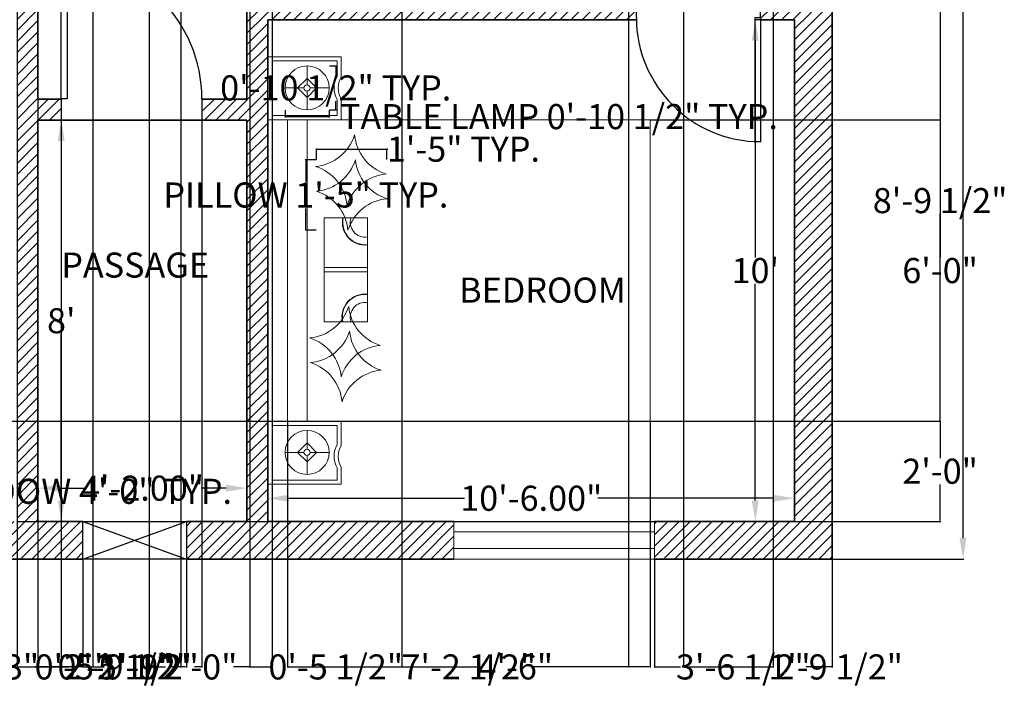
# Model space of a CAD drawing. Units: inches. Extents: x -302 to 383, y -29 to 550.
# Tile 2 of 4: x 147 to 383, y -14 to 149. Entities that reach past the tile are written whole.
import ezdxf

# ---------------------------------------------------------------- set-up
doc = ezdxf.new("R2010")
doc.units = ezdxf.units.IN
doc.header["$MEASUREMENT"] = 0
for name, color, linetype, lineweight in [('A-ANNO-DIMS', 3, 'Continuous', 18), ('A-AREA-IDEN', 2, 'Continuous', 25), ('A-DOOR', 4, 'Continuous', 25), ('A-FURN', 1, 'Continuous', 18), ('A-GLAZ', 2, 'Continuous', 18), ('A-WALL', 7, 'Continuous', 35), ('A-WALL-PATT', 252, 'Continuous', 13)]:
    doc.layers.add(name, color=color, linetype=linetype, lineweight=lineweight)
doc.styles.get("Standard").update_dxf_attribs({"font": 'arial.ttf'})
doc.dimstyles.get("Standard").update_dxf_attribs({"dimtxt": 6, "dimasz": 0.18, "dimexe": 0.18, "dimexo": 0.0625, "dimgap": 0.09, "dimtad": 0, "dimtih": 1, "dimtoh": 1, "dimzin": 0, "dimdsep": 46, "dimlunit": 3, "dimtxsty": 'Standard', "dimcen": 0.09, "dimadec": 0, "dimazin": 0, "dimtfac": 1, "dimtofl": 0, "dimtmove": 0, "dimatfit": 3, "dimfxl": 1, "dimtolj": 1, "dimtzin": 0, "dimarcsym": 0})

# ---------------------------------------------------------------- blocks, each defined once
blk = doc.blocks.new('*U2')
for p, q in [((0, 0), (0, -6)), ((40, 0), (40, -6))]:
    blk.add_line(p, q)
blk.add_lwpolyline([(0, 0), (0, 40), (1.75, 40), (1.75, 0)], close=True)
blk.add_arc((0, 0), 40, 0, 90)
blk = doc.blocks.new('Lamp - Table')
for p, q in [((0, 7), (0, 1)), ((-1, 0), (-7, 0)), ((0, 3), (-3, 0)), ((-3, 0), (0, -3)), ((3, 0), (0, 3)), ((0, -3), (3, 0)), ((1, 0), (7, 0)), ((0, -1), (0, -7))]:
    blk.add_line(p, q)
for radius in [7, 1]:
    blk.add_circle((0, 0), radius)
blk = doc.blocks.new('*D15')
at = {"layer": 'A-ANNO-DIMS', "color": 0, "lineweight": -2, "transparency": 16777216}
for p, q in [((206.7, 29.34), (206.7, 34.99)), ((211.7, 34.81), (253.76, 34.81)), ((327.7, 34.81), (285.64, 34.81)), ((332.7, 29.34), (332.7, 34.99))]:
    blk.add_line(p, q, dxfattribs=at)
at = {"layer": 'A-ANNO-DIMS', "color": 0, "transparency": 16777216}
for points in [[(211.7, 35.64), (211.7, 33.98), (206.7, 34.81)], [(327.7, 35.64), (327.7, 33.98), (332.7, 34.81)]]:
    blk.add_solid(points, dxfattribs=at)
at = {"layer": 'Defpoints', "color": 0, "transparency": 16777216}
for p in [(332.7, 34.81), (206.7, 29.27), (332.7, 29.27)]:
    blk.add_point(p, dxfattribs=at)
at = {"layer": 'A-ANNO-DIMS', "color": 0, "transparency": 16777216, "insert": (269.7, 34.81), "char_height": 6, "attachment_point": 5}
blk.add_mtext('\\A1;10\'-6.00"', dxfattribs=at)
blk = doc.blocks.new('*D16')
at = {"layer": 'A-ANNO-DIMS', "color": 0, "lineweight": -2, "transparency": 16777216}
for p, q in [((332.63, 149.27), (323.11, 149.27)), ((323.29, 144.27), (323.29, 92.43)), ((323.29, 34.27), (323.29, 86.12)), ((332.63, 29.27), (323.11, 29.27))]:
    blk.add_line(p, q, dxfattribs=at)
at = {"layer": 'A-ANNO-DIMS', "color": 0, "transparency": 16777216}
for points in [[(322.45, 144.27), (324.12, 144.27), (323.29, 149.27)], [(322.45, 34.27), (324.12, 34.27), (323.29, 29.27)]]:
    blk.add_solid(points, dxfattribs=at)
at = {"layer": 'Defpoints', "color": 0, "transparency": 16777216}
for p in [(332.7, 149.27), (323.29, 29.27), (332.7, 29.27)]:
    blk.add_point(p, dxfattribs=at)
at = {"layer": 'A-ANNO-DIMS', "color": 0, "transparency": 16777216, "insert": (323.29, 89.27), "char_height": 6, "attachment_point": 5}
blk.add_mtext("\\A1;10'", dxfattribs=at)
blk = doc.blocks.new('*D17')
at = {"layer": 'A-ANNO-DIMS', "color": 0, "lineweight": -2, "transparency": 16777216}
for p, q in [((151.7, 29.34), (151.7, 37.4)), ((156.7, 37.22), (162.69, 37.22)), ((196.7, 37.22), (190.71, 37.22)), ((201.7, 29.34), (201.7, 37.4))]:
    blk.add_line(p, q, dxfattribs=at)
at = {"layer": 'A-ANNO-DIMS', "color": 0, "transparency": 16777216}
for points in [[(156.7, 38.06), (156.7, 36.39), (151.7, 37.22)], [(196.7, 38.06), (196.7, 36.39), (201.7, 37.22)]]:
    blk.add_solid(points, dxfattribs=at)
at = {"layer": 'Defpoints', "color": 0, "transparency": 16777216}
for p in [(201.7, 37.22), (151.7, 29.27), (201.7, 29.27)]:
    blk.add_point(p, dxfattribs=at)
at = {"layer": 'A-ANNO-DIMS', "color": 0, "transparency": 16777216, "insert": (176.7, 37.22), "char_height": 6, "attachment_point": 5}
blk.add_mtext('\\A1;4\'-2.00"', dxfattribs=at)
blk = doc.blocks.new('*D18')
at = {"layer": 'A-ANNO-DIMS', "color": 0, "lineweight": -2, "transparency": 16777216}
for p, q in [((151.76, 125.27), (157.46, 125.27)), ((157.28, 120.27), (157.28, 80.43)), ((157.28, 34.27), (157.28, 74.12)), ((151.76, 29.27), (157.46, 29.27))]:
    blk.add_line(p, q, dxfattribs=at)
at = {"layer": 'A-ANNO-DIMS', "color": 0, "transparency": 16777216}
for points in [[(156.45, 120.27), (158.11, 120.27), (157.28, 125.27)], [(156.45, 34.27), (158.11, 34.27), (157.28, 29.27)]]:
    blk.add_solid(points, dxfattribs=at)
at = {"layer": 'Defpoints', "color": 0, "transparency": 16777216}
for p in [(151.7, 125.27), (151.7, 29.27), (157.28, 29.27)]:
    blk.add_point(p, dxfattribs=at)
at = {"layer": 'A-ANNO-DIMS', "color": 0, "transparency": 16777216, "insert": (157.28, 77.27), "char_height": 6, "attachment_point": 5}
blk.add_mtext("\\A1;8'", dxfattribs=at)
blk = doc.blocks.new('*D22')
at = {"layer": 'A-ANNO-DIMS', "color": 0, "lineweight": -2, "transparency": 16777216}
for p, q in [((341.76, 464.27), (373.16, 464.27)), ((372.98, 459.27), (372.98, 245.43)), ((372.98, 25.27), (372.98, 239.12)), ((341.76, 20.27), (373.16, 20.27))]:
    blk.add_line(p, q, dxfattribs=at)
at = {"layer": 'A-ANNO-DIMS', "color": 0, "transparency": 16777216}
for points in [[(372.15, 459.27), (373.82, 459.27), (372.98, 464.27)], [(372.15, 25.27), (373.82, 25.27), (372.98, 20.27)]]:
    blk.add_solid(points, dxfattribs=at)
at = {"layer": 'Defpoints', "color": 0, "transparency": 16777216}
for p in [(341.7, 464.27), (341.7, 20.27), (372.98, 20.27)]:
    blk.add_point(p, dxfattribs=at)
at = {"layer": 'A-ANNO-DIMS', "color": 0, "transparency": 16777216, "insert": (372.98, 242.27), "char_height": 6, "attachment_point": 5}
blk.add_mtext("\\A1;37'", dxfattribs=at)
blk = doc.blocks.new('WIN-48IN')
blk.add_lwpolyline([(0, 9), (48, 9), (48, 0), (0, 0)], close=True)
for points in [[(0, 6.5), (48, 6.5)], [(0, 2.5), (48, 2.5)]]:
    blk.add_lwpolyline(points)
blk = doc.blocks.new('BED-THROW-PILLOW')
for centre, start, end in [((2.25, 23.4), 275.3318, 342.5062), ((23.4, 21.14), 185.3318, 252.5062), ((0, 2.25), 5.3318, 72.5062), ((21.14, 0), 95.3318, 162.5062)]:
    blk.add_arc(centre, 10.85, start, end)
blk = doc.blocks.new('*D29')
at = {"layer": 'A-ANNO-DIMS', "color": 0, "lineweight": -2, "transparency": 16777216}
for p, q in [((75.47, 29.34), (75.47, 36.65)), ((75.65, 36.47), (123.29, 36.47)), ((123.47, 29.34), (123.47, 36.65)), ((123.47, 36.47), (123.65, 36.47))]:
    blk.add_line(p, q, dxfattribs=at)
at = {"layer": 'A-ANNO-DIMS', "color": 0, "transparency": 16777216}
for points in [[(75.65, 36.5), (75.65, 36.44), (75.47, 36.47)], [(123.29, 36.5), (123.29, 36.44), (123.47, 36.47)]]:
    blk.add_solid(points, dxfattribs=at)
at = {"layer": 'Defpoints', "color": 0, "transparency": 16777216}
for p in [(123.47, 36.47), (75.47, 29.27), (123.47, 29.27)]:
    blk.add_point(p, dxfattribs=at)
at = {"layer": 'A-ANNO-DIMS', "color": 0, "transparency": 16777216, "insert": (161.7, 36.47), "char_height": 6, "attachment_point": 5}
blk.add_mtext('\\A1;WINDOW 4\'-0" TYP.', dxfattribs=at)
blk = doc.blocks.new('*D33')
at = {"layer": 'A-ANNO-DIMS', "color": 0, "lineweight": -2, "transparency": 16777216}
for p, q in [((210.8, 127.61), (210.8, 125.91)), ((221.35, 127.61), (221.35, 125.91)), ((210.98, 126.09), (221.17, 126.09)), ((221.35, 126.09), (221.53, 126.09))]:
    blk.add_line(p, q, dxfattribs=at)
at = {"layer": 'A-ANNO-DIMS', "color": 0, "transparency": 16777216}
for points in [[(210.98, 126.12), (210.98, 126.06), (210.8, 126.09)], [(221.17, 126.12), (221.17, 126.06), (221.35, 126.09)]]:
    blk.add_solid(points, dxfattribs=at)
at = {"layer": 'Defpoints', "color": 0, "transparency": 16777216}
for p in [(210.8, 127.68), (221.35, 127.68), (221.35, 126.09)]:
    blk.add_point(p, dxfattribs=at)
at = {"layer": 'A-ANNO-DIMS', "color": 0, "transparency": 16777216, "insert": (276.32, 126.09), "char_height": 6, "attachment_point": 5}
blk.add_mtext('\\A1;TABLE LAMP 0\'-10 1/2" TYP.', dxfattribs=at)
blk = doc.blocks.new('*D34')
at = {"layer": 'A-ANNO-DIMS', "color": 0, "lineweight": -2, "transparency": 16777216}
for p, q in [((221.41, 138.22), (223.11, 138.22)), ((222.93, 138.04), (222.93, 136.14)), ((222.93, 127.86), (222.93, 129.76)), ((221.41, 127.68), (223.11, 127.68))]:
    blk.add_line(p, q, dxfattribs=at)
at = {"layer": 'A-ANNO-DIMS', "color": 0, "transparency": 16777216}
for points in [[(222.9, 138.04), (222.96, 138.04), (222.93, 138.22)], [(222.9, 127.86), (222.96, 127.86), (222.93, 127.68)]]:
    blk.add_solid(points, dxfattribs=at)
at = {"layer": 'Defpoints', "color": 0, "transparency": 16777216}
for p in [(221.35, 138.22), (222.93, 138.22), (221.35, 127.68)]:
    blk.add_point(p, dxfattribs=at)
at = {"layer": 'A-ANNO-DIMS', "color": 0, "transparency": 16777216, "insert": (222.93, 132.95), "char_height": 6, "attachment_point": 5}
blk.add_mtext('\\A1;0\'-10 1/2" TYP.', dxfattribs=at)
blk = doc.blocks.new('*D35')
at = {"layer": 'A-ANNO-DIMS', "color": 0, "lineweight": -2, "transparency": 16777216}
for p, q in [((218.26, 115.78), (215.61, 115.78)), ((215.79, 115.6), (215.79, 110.54)), ((215.79, 99.08), (215.79, 104.15)), ((218.26, 98.9), (215.61, 98.9))]:
    blk.add_line(p, q, dxfattribs=at)
at = {"layer": 'A-ANNO-DIMS', "color": 0, "transparency": 16777216}
for points in [[(215.76, 115.6), (215.82, 115.6), (215.79, 115.78)], [(215.76, 99.08), (215.82, 99.08), (215.79, 98.9)]]:
    blk.add_solid(points, dxfattribs=at)
at = {"layer": 'Defpoints', "color": 0, "transparency": 16777216}
for p in [(215.79, 115.78), (218.32, 115.78), (218.32, 98.9)]:
    blk.add_point(p, dxfattribs=at)
at = {"layer": 'A-ANNO-DIMS', "color": 0, "transparency": 16777216, "insert": (215.79, 107.34), "char_height": 6, "attachment_point": 5}
blk.add_mtext('\\A1;PILLOW 1\'-5" TYP.', dxfattribs=at)
blk = doc.blocks.new('*D36')
at = {"layer": 'A-ANNO-DIMS', "color": 0, "lineweight": -2, "transparency": 16777216}
for p, q in [((218.32, 115.84), (218.32, 118.49)), ((218.5, 118.31), (235.01, 118.31)), ((235.19, 115.84), (235.19, 118.49)), ((235.19, 118.31), (235.37, 118.31))]:
    blk.add_line(p, q, dxfattribs=at)
at = {"layer": 'A-ANNO-DIMS', "color": 0, "transparency": 16777216}
for points in [[(218.5, 118.34), (218.5, 118.28), (218.32, 118.31)], [(235.01, 118.34), (235.01, 118.28), (235.19, 118.31)]]:
    blk.add_solid(points, dxfattribs=at)
at = {"layer": 'Defpoints', "color": 0, "transparency": 16777216}
for p in [(235.19, 118.31), (218.32, 115.78), (235.19, 115.78)]:
    blk.add_point(p, dxfattribs=at)
at = {"layer": 'A-ANNO-DIMS', "color": 0, "transparency": 16777216, "insert": (253.47, 118.31), "char_height": 6, "attachment_point": 5}
blk.add_mtext('\\A1;1\'-5" TYP.', dxfattribs=at)
blk = doc.blocks.new('*D38')
at = {"layer": 'A-ANNO-DIMS', "color": 0, "lineweight": -2, "transparency": 16777216}
for p, q in [((123.47, 20.21), (123.47, -5.71)), ((162.44, 20.21), (162.44, -5.71)), ((123.65, -5.53), (134.89, -5.53)), ((162.26, -5.53), (151.02, -5.53))]:
    blk.add_line(p, q, dxfattribs=at)
at = {"layer": 'A-ANNO-DIMS', "color": 0, "transparency": 16777216}
for points in [[(123.65, -5.5), (123.65, -5.56), (123.47, -5.53)], [(162.26, -5.5), (162.26, -5.56), (162.44, -5.53)]]:
    blk.add_solid(points, dxfattribs=at)
at = {"layer": 'Defpoints', "color": 0, "transparency": 16777216}
for p in [(123.47, 20.27), (162.44, 20.27), (162.44, -5.53)]:
    blk.add_point(p, dxfattribs=at)
at = {"layer": 'A-ANNO-DIMS', "color": 0, "transparency": 16777216, "insert": (142.95, -5.53), "char_height": 6, "attachment_point": 5}
blk.add_mtext('\\A1;3\'-3"', dxfattribs=at)
blk = doc.blocks.new('*D39')
at = {"layer": 'A-ANNO-DIMS', "color": 0, "lineweight": -2, "transparency": 16777216}
for p, q in [((162.44, 20.21), (162.44, -5.71)), ((187.2, 20.21), (187.2, -5.71)), ((162.62, -5.53), (166.7, -5.53)), ((187.02, -5.53), (182.94, -5.53))]:
    blk.add_line(p, q, dxfattribs=at)
at = {"layer": 'A-ANNO-DIMS', "color": 0, "transparency": 16777216}
for points in [[(162.62, -5.5), (162.62, -5.56), (162.44, -5.53)], [(187.02, -5.5), (187.02, -5.56), (187.2, -5.53)]]:
    blk.add_solid(points, dxfattribs=at)
at = {"layer": 'Defpoints', "color": 0, "transparency": 16777216}
for p in [(162.44, 20.27), (187.2, 20.27), (187.2, -5.53)]:
    blk.add_point(p, dxfattribs=at)
at = {"layer": 'A-ANNO-DIMS', "color": 0, "transparency": 16777216, "insert": (174.82, -5.53), "char_height": 6, "attachment_point": 5}
blk.add_mtext('\\A1;2\'-1"', dxfattribs=at)
blk = doc.blocks.new('*D40')
at = {"layer": 'A-ANNO-DIMS', "color": 0, "lineweight": -2, "transparency": 16777216}
for p, q in [((299.16, 20.21), (299.16, -5.71)), ((341.7, 20.21), (341.7, -5.71)), ((299.34, -5.53), (305.37, -5.53)), ((341.52, -5.53), (335.48, -5.53))]:
    blk.add_line(p, q, dxfattribs=at)
at = {"layer": 'A-ANNO-DIMS', "color": 0, "transparency": 16777216}
for points in [[(299.34, -5.5), (299.34, -5.56), (299.16, -5.53)], [(341.52, -5.5), (341.52, -5.56), (341.7, -5.53)]]:
    blk.add_solid(points, dxfattribs=at)
at = {"layer": 'Defpoints', "color": 0, "transparency": 16777216}
for p in [(299.16, 20.27), (341.7, 20.27), (341.7, -5.53)]:
    blk.add_point(p, dxfattribs=at)
at = {"layer": 'A-ANNO-DIMS', "color": 0, "transparency": 16777216, "insert": (320.43, -5.53), "char_height": 6, "attachment_point": 5}
blk.add_mtext('\\A1;3\'-6 1/2"', dxfattribs=at)
blk = doc.blocks.new('*D50')
at = {"layer": 'A-ANNO-DIMS', "color": 0, "lineweight": -2, "transparency": 16777216}
for p, q in [((178.34, 359.21), (178.34, -5.71)), ((202.4, 359.21), (202.4, -5.71)), ((178.52, -5.53), (182.25, -5.53)), ((202.22, -5.53), (198.48, -5.53))]:
    blk.add_line(p, q, dxfattribs=at)
at = {"layer": 'A-ANNO-DIMS', "color": 0, "transparency": 16777216}
for points in [[(178.52, -5.5), (178.52, -5.56), (178.34, -5.53)], [(202.22, -5.5), (202.22, -5.56), (202.4, -5.53)]]:
    blk.add_solid(points, dxfattribs=at)
at = {"layer": 'Defpoints', "color": 0, "transparency": 16777216}
for p in [(178.34, 359.27), (202.4, 359.27), (202.4, -5.53)]:
    blk.add_point(p, dxfattribs=at)
at = {"layer": 'A-ANNO-DIMS', "color": 0, "transparency": 16777216, "insert": (190.37, -5.53), "char_height": 6, "attachment_point": 5}
blk.add_mtext('\\A1;2\'-0"', dxfattribs=at)
blk = doc.blocks.new('*D52')
at = {"layer": 'A-ANNO-DIMS', "color": 0, "lineweight": -2, "transparency": 16777216}
for p, q in [((157.23, 130.21), (157.23, -5.71)), ((190.92, 130.21), (190.92, -5.71)), ((157.41, -5.53), (158.97, -5.53)), ((190.74, -5.53), (189.18, -5.53))]:
    blk.add_line(p, q, dxfattribs=at)
at = {"layer": 'A-ANNO-DIMS', "color": 0, "transparency": 16777216}
for points in [[(157.41, -5.5), (157.41, -5.56), (157.23, -5.53)], [(190.74, -5.5), (190.74, -5.56), (190.92, -5.53)]]:
    blk.add_solid(points, dxfattribs=at)
at = {"layer": 'Defpoints', "color": 0, "transparency": 16777216}
for p in [(157.23, 130.27), (190.92, 130.27), (190.92, -5.53)]:
    blk.add_point(p, dxfattribs=at)
at = {"layer": 'A-ANNO-DIMS', "color": 0, "transparency": 16777216, "insert": (174.08, -5.53), "char_height": 6, "attachment_point": 5}
blk.add_mtext('\\A1;2\'-9 1/2"', dxfattribs=at)
blk = doc.blocks.new('*D58')
at = {"layer": 'A-ANNO-DIMS', "color": 0, "lineweight": -2, "transparency": 16777216}
for p, q in [((50.76, 158.73), (367.68, 158.73)), ((367.5, 158.55), (367.5, 109.19)), ((367.5, 53.45), (367.5, 102.81)), ((50.76, 53.27), (367.68, 53.27))]:
    blk.add_line(p, q, dxfattribs=at)
at = {"layer": 'A-ANNO-DIMS', "color": 0, "transparency": 16777216}
for points in [[(367.47, 158.55), (367.53, 158.55), (367.5, 158.73)], [(367.47, 53.45), (367.53, 53.45), (367.5, 53.27)]]:
    blk.add_solid(points, dxfattribs=at)
at = {"layer": 'Defpoints', "color": 0, "transparency": 16777216}
for p in [(50.7, 158.73), (367.5, 158.73), (50.7, 53.27)]:
    blk.add_point(p, dxfattribs=at)
at = {"layer": 'A-ANNO-DIMS', "color": 0, "transparency": 16777216, "insert": (367.5, 106), "char_height": 6, "attachment_point": 5}
blk.add_mtext('\\A1;8\'-9 1/2"', dxfattribs=at)
blk = doc.blocks.new('*D60')
at = {"layer": 'A-ANNO-DIMS', "color": 0, "lineweight": -2, "transparency": 16777216}
for p, q in [((164.84, 447.21), (164.84, -5.71)), ((185.84, 447.21), (185.84, -5.71)), ((165.02, -5.53), (167.56, -5.53)), ((185.66, -5.53), (183.12, -5.53))]:
    blk.add_line(p, q, dxfattribs=at)
at = {"layer": 'A-ANNO-DIMS', "color": 0, "transparency": 16777216}
for points in [[(165.02, -5.5), (165.02, -5.56), (164.84, -5.53)], [(185.66, -5.5), (185.66, -5.56), (185.84, -5.53)]]:
    blk.add_solid(points, dxfattribs=at)
at = {"layer": 'Defpoints', "color": 0, "transparency": 16777216}
for p in [(164.84, 447.27), (185.84, 447.27), (185.84, -5.53)]:
    blk.add_point(p, dxfattribs=at)
at = {"layer": 'A-ANNO-DIMS', "color": 0, "transparency": 16777216, "insert": (175.34, -5.53), "char_height": 6, "attachment_point": 5}
blk.add_mtext('\\A1;1\'-9"', dxfattribs=at)
blk = doc.blocks.new('*D64')
at = {"layer": 'A-ANNO-DIMS', "color": 0, "lineweight": -2, "transparency": 16777216}
for p, q in [((238.76, 232.51), (238.76, -5.71)), ((292.99, 232.51), (292.99, -5.71)), ((238.94, -5.53), (257.69, -5.53)), ((292.81, -5.53), (274.06, -5.53))]:
    blk.add_line(p, q, dxfattribs=at)
at = {"layer": 'A-ANNO-DIMS', "color": 0, "transparency": 16777216}
for points in [[(238.94, -5.5), (238.94, -5.56), (238.76, -5.53)], [(292.81, -5.5), (292.81, -5.56), (292.99, -5.53)]]:
    blk.add_solid(points, dxfattribs=at)
at = {"layer": 'Defpoints', "color": 0, "transparency": 16777216}
for p in [(238.76, 232.57), (292.99, 232.57), (292.99, -5.53)]:
    blk.add_point(p, dxfattribs=at)
at = {"layer": 'A-ANNO-DIMS', "color": 0, "transparency": 16777216, "insert": (265.88, -5.53), "char_height": 6, "attachment_point": 5}
blk.add_mtext('\\A1;4\'-6"', dxfattribs=at)
blk = doc.blocks.new('*D66')
at = {"layer": 'A-ANNO-DIMS', "color": 0, "lineweight": -2, "transparency": 16777216}
for p, q in [((211.41, 53.15), (211.41, -5.71)), ((298.12, 53.15), (298.12, -5.71)), ((211.59, -5.53), (239.73, -5.53)), ((297.94, -5.53), (269.79, -5.53))]:
    blk.add_line(p, q, dxfattribs=at)
at = {"layer": 'A-ANNO-DIMS', "color": 0, "transparency": 16777216}
for points in [[(211.59, -5.5), (211.59, -5.56), (211.41, -5.53)], [(297.94, -5.5), (297.94, -5.56), (298.12, -5.53)]]:
    blk.add_solid(points, dxfattribs=at)
at = {"layer": 'Defpoints', "color": 0, "transparency": 16777216}
for p in [(211.41, 53.21), (298.12, 53.21), (298.12, -5.53)]:
    blk.add_point(p, dxfattribs=at)
at = {"layer": 'A-ANNO-DIMS', "color": 0, "transparency": 16777216, "insert": (254.76, -5.53), "char_height": 6, "attachment_point": 5}
blk.add_mtext('\\A1;7\'-2 1/2"', dxfattribs=at)
blk = doc.blocks.new('*D67')
at = {"layer": 'A-ANNO-DIMS', "color": 0, "lineweight": -2, "transparency": 16777216}
for p, q in [((298.18, 125.33), (367.68, 125.33)), ((367.5, 125.15), (367.5, 92.43)), ((367.5, 53.39), (367.5, 86.12)), ((298.18, 53.21), (367.68, 53.21))]:
    blk.add_line(p, q, dxfattribs=at)
at = {"layer": 'A-ANNO-DIMS', "color": 0, "transparency": 16777216}
for points in [[(367.47, 125.15), (367.53, 125.15), (367.5, 125.33)], [(367.47, 53.39), (367.53, 53.39), (367.5, 53.21)]]:
    blk.add_solid(points, dxfattribs=at)
at = {"layer": 'Defpoints', "color": 0, "transparency": 16777216}
for p in [(298.12, 125.33), (367.5, 125.33), (298.12, 53.21)]:
    blk.add_point(p, dxfattribs=at)
at = {"layer": 'A-ANNO-DIMS', "color": 0, "transparency": 16777216, "insert": (367.5, 89.27), "char_height": 6, "attachment_point": 5}
blk.add_mtext('\\A1;6\'-0"', dxfattribs=at)
blk = doc.blocks.new('*D69')
at = {"layer": 'A-ANNO-DIMS', "color": 0, "lineweight": -2, "transparency": 16777216}
for p, q in [((146.76, 53.27), (367.68, 53.27)), ((367.5, 53.09), (367.5, 44.43)), ((367.5, 29.45), (367.5, 38.12)), ((146.76, 29.27), (367.68, 29.27))]:
    blk.add_line(p, q, dxfattribs=at)
at = {"layer": 'A-ANNO-DIMS', "color": 0, "transparency": 16777216}
for points in [[(367.47, 53.09), (367.53, 53.09), (367.5, 53.27)], [(367.47, 29.45), (367.53, 29.45), (367.5, 29.27)]]:
    blk.add_solid(points, dxfattribs=at)
at = {"layer": 'Defpoints', "color": 0, "transparency": 16777216}
for p in [(146.7, 53.27), (367.5, 53.27), (146.7, 29.27)]:
    blk.add_point(p, dxfattribs=at)
at = {"layer": 'A-ANNO-DIMS', "color": 0, "transparency": 16777216, "insert": (367.5, 41.27), "char_height": 6, "attachment_point": 5}
blk.add_mtext('\\A1;2\'-0"', dxfattribs=at)
blk = doc.blocks.new('*D71')
at = {"layer": 'A-ANNO-DIMS', "color": 0, "lineweight": -2, "transparency": 16777216}
for p, q in [((146.7, 358.81), (146.7, -5.71)), ((151.7, 354.21), (151.7, -5.71)), ((146.88, -5.53), (151.52, -5.53)), ((151.7, -5.53), (151.88, -5.53))]:
    blk.add_line(p, q, dxfattribs=at)
at = {"layer": 'A-ANNO-DIMS', "color": 0, "transparency": 16777216}
for points in [[(146.88, -5.5), (146.88, -5.56), (146.7, -5.53)], [(151.52, -5.5), (151.52, -5.56), (151.7, -5.53)]]:
    blk.add_solid(points, dxfattribs=at)
at = {"layer": 'Defpoints', "color": 0, "transparency": 16777216}
for p in [(146.7, 358.87), (151.7, 354.27), (151.7, -5.53)]:
    blk.add_point(p, dxfattribs=at)
at = {"layer": 'A-ANNO-DIMS', "color": 0, "transparency": 16777216, "insert": (159.94, -5.53), "char_height": 6, "attachment_point": 5}
blk.add_mtext('\\A1;0\'-5"', dxfattribs=at)
blk = doc.blocks.new('*D72')
at = {"layer": 'A-ANNO-DIMS', "color": 0, "lineweight": -2, "transparency": 16777216}
for p, q in [((202.4, 354.21), (202.4, -5.71)), ((207.7, 354.21), (207.7, -5.71)), ((202.58, -5.53), (207.52, -5.53)), ((207.7, -5.53), (207.88, -5.53))]:
    blk.add_line(p, q, dxfattribs=at)
at = {"layer": 'A-ANNO-DIMS', "color": 0, "transparency": 16777216}
for points in [[(202.58, -5.5), (202.58, -5.56), (202.4, -5.53)], [(207.52, -5.5), (207.52, -5.56), (207.7, -5.53)]]:
    blk.add_solid(points, dxfattribs=at)
at = {"layer": 'Defpoints', "color": 0, "transparency": 16777216}
for p in [(202.4, 354.27), (207.7, 354.27), (207.7, -5.53)]:
    blk.add_point(p, dxfattribs=at)
at = {"layer": 'A-ANNO-DIMS', "color": 0, "transparency": 16777216, "insert": (222.93, -5.53), "char_height": 6, "attachment_point": 5}
blk.add_mtext('\\A1;0\'-5 1/2"', dxfattribs=at)
blk = doc.blocks.new('*D76')
at = {"layer": 'A-ANNO-DIMS', "color": 0, "lineweight": -2, "transparency": 16777216}
for p, q in [((151.7, 125.21), (151.7, -5.71)), ((157.23, 125.21), (157.23, -5.71)), ((151.88, -5.53), (157.05, -5.53)), ((157.23, -5.53), (157.41, -5.53))]:
    blk.add_line(p, q, dxfattribs=at)
at = {"layer": 'A-ANNO-DIMS', "color": 0, "transparency": 16777216}
for points in [[(151.88, -5.5), (151.88, -5.56), (151.7, -5.53)], [(157.05, -5.5), (157.05, -5.56), (157.23, -5.53)]]:
    blk.add_solid(points, dxfattribs=at)
at = {"layer": 'Defpoints', "color": 0, "transparency": 16777216}
for p in [(151.7, 125.27), (157.23, 125.27), (157.23, -5.53)]:
    blk.add_point(p, dxfattribs=at)
at = {"layer": 'A-ANNO-DIMS', "color": 0, "transparency": 16777216, "insert": (172.47, -5.53), "char_height": 6, "attachment_point": 5}
blk.add_mtext('\\A1;0\'-5 1/2"', dxfattribs=at)
blk = doc.blocks.new('*D77')
at = {"layer": 'A-ANNO-DIMS', "color": 0, "lineweight": -2, "transparency": 16777216}
for p, q in [((306.08, 275.31), (306.08, -5.71)), ((327.55, 275.31), (327.55, -5.71)), ((306.26, -5.53), (327.37, -5.53)), ((327.55, -5.53), (327.73, -5.53))]:
    blk.add_line(p, q, dxfattribs=at)
at = {"layer": 'A-ANNO-DIMS', "color": 0, "transparency": 16777216}
for points in [[(306.26, -5.5), (306.26, -5.56), (306.08, -5.53)], [(327.37, -5.5), (327.37, -5.56), (327.55, -5.53)]]:
    blk.add_solid(points, dxfattribs=at)
at = {"layer": 'Defpoints', "color": 0, "transparency": 16777216}
for p in [(306.08, 275.38), (327.55, 275.38), (327.55, -5.53)]:
    blk.add_point(p, dxfattribs=at)
at = {"layer": 'A-ANNO-DIMS', "color": 0, "transparency": 16777216, "insert": (342.5, -5.53), "char_height": 6, "attachment_point": 5}
blk.add_mtext('\\A1;1\'-9 1/2"', dxfattribs=at)

msp = doc.modelspace()

# ---------------------------------------------------------------- hatches: boundary and pattern name
at = {"layer": 'A-WALL-PATT'}
h = msp.add_hatch(dxfattribs=at)
h.set_pattern_fill('ANSI31', color=256, scale=15)
h.paths.add_polyline_path([(201.697, 29.273), (187.202, 29.273), (187.202, 20.273), (251.158, 20.273), (251.158, 29.273), (206.697, 29.273), (206.697, 149.273), (294.846, 149.273, -0.0045588), (294.841, 149.815), (294.841, 154.273), (201.697, 154.273), (201.697, 130.273), (190.923, 130.273), (190.923, 125.273), (201.697, 125.273)])
h.paths.add_polyline_path([(341.697, 154.273), (332.697, 154.273), (324.561, 154.273), (324.561, 149.815), (324.561, 149.273), (332.697, 149.273), (332.697, 29.273), (299.158, 29.273), (299.158, 20.273), (341.697, 20.273)])
h.paths.add_polyline_path([(75.47, 20.273), (75.47, 29.273), (26.697, 29.273), (26.697, 89.142), (17.697, 89.142), (17.697, 20.273)])
h.paths.add_polyline_path([(26.697, 221.273), (146.697, 221.273), (146.697, 217.323), (147.147, 217.323), (151.697, 217.323), (151.697, 226.273), (26.697, 226.273), (26.697, 248.984), (17.697, 248.984), (17.697, 137.142), (26.697, 137.142)])
h.paths.add_polyline_path([(17.697, 284.934), (26.697, 284.934), (26.697, 306.273), (151.697, 306.273), (151.697, 317.511), (147.338, 317.511), (146.697, 317.511), (146.697, 311.273), (26.697, 311.273), (26.697, 377.22), (17.697, 377.22)])
h.paths.add_polyline_path([(341.697, 376.674), (332.697, 376.674), (332.697, 311.273), (212.697, 311.273), (212.697, 317.511), (212.055, 317.511), (207.697, 317.511), (207.697, 306.273), (332.697, 306.273), (332.697, 214.273), (341.697, 214.273)])
h.paths.add_polyline_path([(207.697, 455.273), (207.697, 359.273), (202.395, 359.273), (202.395, 357.888), (202.395, 354.273), (207.697, 354.273), (207.697, 346.57), (212.055, 346.57, -0.0055163), (212.697, 346.563), (212.697, 455.273), (332.697, 455.273), (332.697, 424.674), (341.697, 424.674), (341.697, 464.273), (188.075, 464.273), (188.075, 455.273)])
h.paths.add_polyline_path([(17.697, 464.273), (17.697, 425.22), (26.697, 425.22), (26.697, 455.273), (146.697, 455.273), (146.697, 346.563, -0.0055163), (147.338, 346.57), (151.697, 346.57), (151.697, 354.273), (178.3, 354.273), (178.3, 357.888, -0.0143868), (178.34, 359.273), (151.697, 359.273), (151.697, 455.273), (162.634, 455.273), (162.634, 464.273)])
h = msp.add_hatch(dxfattribs=at)
h.set_pattern_fill('ANSI31', color=256, scale=15)
h.paths.add_polyline_path([(151.697, 186.995), (147.147, 186.995, -0.0037161), (146.697, 186.998), (146.697, 29.273), (123.47, 29.273), (123.47, 20.273), (162.437, 20.273), (162.437, 29.273), (151.697, 29.273), (151.697, 125.273), (157.23, 125.273), (157.23, 130.273), (151.697, 130.273)])

# ---------------------------------------------------------------- linework, layer by layer
at = {"layer": 'A-DOOR'}
for p, q in [((162.437, 29.273), (187.202, 20.273)), ((162.437, 20.273), (187.202, 29.273))]:
    msp.add_line(p, q, dxfattribs=at)
msp.add_lwpolyline([(162.437, 29.273), (187.202, 29.273), (187.202, 20.273), (162.437, 20.273)], close=True, dxfattribs=at)
at = {"layer": 'A-FURN'}
for p, q in [((224.252, 140.4), (224.252, 135.473)), ((224.252, 130.425), (224.252, 125.332)), ((211.409, 125.332), (211.409, 53.215)), ((216.119, 125.332), (216.119, 53.215)), ((220.173, 89.964), (230.516, 89.964)), ((220.173, 88.964), (230.516, 88.964))]:
    msp.add_line(p, q, dxfattribs=at)
for points in [[(224.252, 140.4), (206.697, 140.4), (206.697, 125.332), (224.252, 125.332)], [(223.252, 135.747), (223.252, 139.4), (207.697, 139.4), (207.697, 126.332), (223.252, 126.332), (223.252, 130.151)], [(224.252, 42.321), (224.252, 38.146), (206.697, 38.146), (206.697, 53.215), (224.252, 53.215), (224.252, 47.361)], [(223.252, 42.048), (223.252, 39.146), (207.697, 39.146), (207.697, 52.215), (223.252, 52.215), (223.252, 47.634)]]:
    msp.add_lwpolyline(points, dxfattribs=at)
for points in [[(206.697, 125.332), (298.118, 125.332), (298.118, 53.215), (206.697, 53.215)], [(220.173, 101.894), (230.516, 101.894), (230.516, 77.034), (220.173, 77.034)]]:
    msp.add_lwpolyline(points, close=True, dxfattribs=at)
for centre, radius, start, end in [((228.262, 132.949), 5.738, 150.81881, 209.18119), ((228.262, 132.949), 4.738, 147.81122, 212.18878), ((229.945, 100.793), 5.43, 168.30204, 276.03359), ((229.945, 100.793), 5.33, 168.30204, 276.03359), ((229.945, 100.793), 3.53, 161.82799, 279.30448), ((229.945, 78.136), 5.53, 84.0759, 191.48354), ((229.945, 78.136), 5.43, 83.96641, 191.69796), ((229.945, 78.136), 3.53, 80.69552, 198.17201), ((228.265, 44.841), 5.738, 150.87624, 209.12376), ((228.265, 44.841), 4.738, 147.87487, 212.12513)]:
    msp.add_arc(centre, radius, start, end, dxfattribs=at)
at = {"layer": 'A-WALL'}
for points in [[(151.697, 226.273), (151.697, 130.273)], [(201.697, 130.273), (201.697, 154.273)], [(299.158, 20.273), (341.697, 20.273), (341.697, 154.273)], [(206.697, 29.273), (206.697, 149.273)], [(206.697, 149.273), (294.846, 149.273)], [(324.561, 149.273), (332.697, 149.273)], [(332.697, 29.273), (332.697, 149.273)], [(151.697, 130.273), (157.23, 130.273)], [(190.923, 130.273), (201.697, 130.273)], [(151.697, 125.273), (201.697, 125.273)], [(151.697, 125.273), (151.697, 29.273)], [(201.697, 29.273), (201.697, 125.273)], [(151.697, 29.273), (162.437, 29.273)], [(187.202, 29.273), (201.697, 29.273)], [(206.697, 29.273), (251.158, 29.273)], [(299.158, 29.273), (332.697, 29.273)], [(123.47, 20.273), (162.437, 20.273)], [(187.202, 20.273), (251.158, 20.273)]]:
    msp.add_lwpolyline(points, dxfattribs=at)

# ---------------------------------------------------------------- block references
at = {"layer": 'A-DOOR', "xscale": 0.8423175493774062, "yscale": 0.8423175493774062, "zscale": 0.8423175493774062}
msp.add_blockref('*U2', (157.23, 130.327), dxfattribs=at)
at = {"layer": 'A-DOOR', "xscale": 0.7430126011318324, "yscale": 0.7430126011318324, "zscale": 0.7430126011318324, "rotation": 180}
msp.add_blockref('*U2', (324.561, 149.815), dxfattribs=at)
at = {"layer": 'A-FURN', "xscale": 0.7534115597809233, "yscale": 0.7534115597809233, "zscale": 0.7534115597809233}
for p in [(216.076, 132.949), (216.076, 45.781)]:
    msp.add_blockref('Lamp - Table', p, dxfattribs=at)
at = {"layer": 'A-FURN'}
for p, rotation in [((238.241, 101.565), 90.00000000000357), ((236.833, 60.569), 90.00000000000357), ((237.046, 54.648), 90.00000000000104)]:
    msp.add_blockref('BED-THROW-PILLOW', p, dxfattribs=dict(at, rotation=rotation))
msp.add_blockref('BED-THROW-PILLOW', (215.058, 95.644), dxfattribs=at)
at = {"layer": 'A-GLAZ'}
msp.add_blockref('WIN-48IN', (251.158, 20.273), dxfattribs=at)

# ---------------------------------------------------------------- texts
at = {"layer": 'A-AREA-IDEN', "char_height": 6, "attachment_point": 1}
for s, width, insert in [('{PASSAGE}', 74.36308, (157.281, 93.58)), ('{BEDROOM}', 101.54109, (252.452, 87.595))]:
    msp.add_mtext_dynamic_manual_height_columns(s, width=width, gutter_width=1, heights=[0], dxfattribs=dict(at, insert=insert))

# ---------------------------------------------------------------- dimensions: what is measured, and where the dimension line sits
at = {"layer": 'A-ANNO-DIMS'}
for base, p1, p2, override, picture, middle in [((372.983, 20.273), (341.697, 464.273), (341.697, 20.273), {"dimasz": 5, "dimclrd": 0, "dimclre": 0, "dimclrt": 0}, '*D22', (372.983, 242.273)), ((367.497, 158.726), (50.697, 53.273), (50.697, 158.726), {"dimdec": 1, "dimlfac": 1, "dimrnd": 0, "dimzin": 1, "dimdsep": 46, "dimlunit": 4, "dimfrac": 2}, '*D58', (367.497, 106)), ((323.287, 29.273), (332.697, 149.273), (332.697, 29.273), {"dimasz": 5, "dimclrd": 0, "dimclre": 0, "dimclrt": 0}, '*D16', (323.287, 89.273)), ((157.281, 29.273), (151.697, 125.273), (151.697, 29.273), {"dimasz": 5, "dimclrd": 0, "dimclre": 0, "dimclrt": 0}, '*D18', (157.281, 77.273)), ((367.497, 125.332), (298.118, 53.215), (298.118, 125.332), {"dimdec": 1, "dimlfac": 1, "dimrnd": 0, "dimzin": 1, "dimdsep": 46, "dimlunit": 4, "dimfrac": 2}, '*D67', (367.497, 89.273)), ((367.497, 53.273), (146.697, 29.273), (146.697, 53.273), {"dimdec": 1, "dimlfac": 1, "dimrnd": 0, "dimzin": 1, "dimdsep": 46, "dimlunit": 4, "dimfrac": 2}, '*D69', (367.497, 41.273))]:
    dim = msp.add_linear_dim(base=base, p1=p1, p2=p2, angle=90, dimstyle='Standard', override=override, dxfattribs=at)
    dim.commit()
    dim.dimension.update_dxf_attribs({"geometry": picture, "text_midpoint": middle})
for base, p1, p2, override, picture, middle in [((185.841, -5.527), (164.841, 447.273), (185.841, 447.273), {"dimdec": 1, "dimlfac": 1, "dimrnd": 0, "dimzin": 1, "dimdsep": 46, "dimlunit": 4, "dimfrac": 2}, '*D60', (175.341, -5.527)), ((151.697, -5.527), (146.697, 358.869), (151.697, 354.273), {"dimdec": 1, "dimlfac": 1, "dimrnd": 0, "dimzin": 1, "dimdsep": 46, "dimlunit": 4, "dimfrac": 2}, '*D71', (159.941, -5.527)), ((202.395, -5.527), (178.34, 359.273), (202.395, 359.273), {"dimdec": 1, "dimlfac": 1, "dimrnd": 0, "dimzin": 1, "dimdsep": 46, "dimlunit": 4, "dimfrac": 2}, '*D50', (190.367, -5.527)), ((207.697, -5.527), (202.395, 354.273), (207.697, 354.273), {"dimdec": 1, "dimlfac": 1, "dimrnd": 0, "dimzin": 1, "dimdsep": 46, "dimlunit": 4, "dimfrac": 2}, '*D72', (222.932, -5.527)), ((327.545, -5.527), (306.081, 275.376), (327.545, 275.376), {"dimdec": 1, "dimlfac": 1, "dimrnd": 0, "dimzin": 1, "dimdsep": 46, "dimlunit": 4, "dimfrac": 2}, '*D77', (342.498, -5.527)), ((292.993, -5.527), (238.759, 232.573), (292.993, 232.573), {"dimdec": 1, "dimlfac": 1, "dimrnd": 0, "dimzin": 1, "dimdsep": 46, "dimlunit": 4, "dimfrac": 2}, '*D64', (265.876, -5.527)), ((190.923, -5.527), (157.23, 130.273), (190.923, 130.273), {"dimdec": 1, "dimlfac": 1, "dimrnd": 0, "dimzin": 1, "dimdsep": 46, "dimlunit": 4, "dimfrac": 2}, '*D52', (174.076, -5.527)), ((157.23, -5.527), (151.697, 125.273), (157.23, 125.273), {"dimdec": 1, "dimlfac": 1, "dimrnd": 0, "dimzin": 1, "dimdsep": 46, "dimlunit": 4, "dimfrac": 2}, '*D76', (172.465, -5.527)), ((298.118, -5.527), (211.409, 53.215), (298.118, 53.215), {"dimdec": 1, "dimlfac": 1, "dimrnd": 0, "dimzin": 1, "dimdsep": 46, "dimlunit": 4, "dimfrac": 2}, '*D66', (254.763, -5.527)), ((201.697, 37.224), (151.697, 29.273), (201.697, 29.273), {"dimasz": 5, "dimclrd": 0, "dimclre": 0, "dimclrt": 0}, '*D17', (176.697, 37.224)), ((332.697, 34.812), (206.697, 29.273), (332.697, 29.273), {"dimasz": 5, "dimclrd": 0, "dimclre": 0, "dimclrt": 0}, '*D15', (269.697, 34.812)), ((162.437, -5.527), (123.47, 20.273), (162.437, 20.273), {"dimdec": 1, "dimlfac": 1, "dimrnd": 0, "dimzin": 1, "dimdsep": 46, "dimlunit": 4, "dimfrac": 2}, '*D38', (142.954, -5.527)), ((187.202, -5.527), (162.437, 20.273), (187.202, 20.273), {"dimdec": 1, "dimlfac": 1, "dimrnd": 0, "dimzin": 1, "dimdsep": 46, "dimlunit": 4, "dimfrac": 2}, '*D39', (174.82, -5.527)), ((341.697, -5.527), (299.158, 20.273), (341.697, 20.273), {"dimdec": 1, "dimlfac": 1, "dimrnd": 0, "dimzin": 1, "dimdsep": 46, "dimlunit": 4, "dimfrac": 2}, '*D40', (320.427, -5.527))]:
    dim = msp.add_linear_dim(base=base, p1=p1, p2=p2, dimstyle='Standard', override=override, dxfattribs=at)
    dim.commit()
    dim.dimension.update_dxf_attribs({"geometry": picture, "text_midpoint": middle})
for base, p1, p2, text, picture, middle in [((221.35, 126.093), (210.802, 127.675), (221.35, 127.675), 'TABLE LAMP <> TYP.', '*D33', (276.322, 126.093)), ((235.193, 118.31), (218.318, 115.779), (235.193, 115.779), '<> TYP.', '*D36', (253.467, 118.31)), ((123.47, 36.473), (75.47, 29.273), (123.47, 29.273), 'WINDOW <> TYP.', '*D29', (161.703, 36.473))]:
    dim = msp.add_linear_dim(base=base, p1=p1, p2=p2, text=text, dimstyle='Standard', override={"dimdec": 1, "dimlfac": 1, "dimrnd": 0, "dimzin": 1, "dimdsep": 46, "dimlunit": 4, "dimfrac": 2}, dxfattribs=at)
    dim.commit()
    dim.dimension.update_dxf_attribs({"geometry": picture, "text_midpoint": middle})
for base, p1, p2, text, picture, middle in [((222.932, 138.223), (221.35, 127.675), (221.35, 138.223), '<> TYP.', '*D34', (222.932, 132.949)), ((215.787, 115.779), (218.318, 98.904), (218.318, 115.779), 'PILLOW <> TYP.', '*D35', (215.787, 107.342))]:
    dim = msp.add_linear_dim(base=base, p1=p1, p2=p2, angle=90, text=text, dimstyle='Standard', override={"dimdec": 1, "dimlfac": 1, "dimrnd": 0, "dimzin": 1, "dimdsep": 46, "dimlunit": 4, "dimfrac": 2}, dxfattribs=at)
    dim.commit()
    dim.dimension.update_dxf_attribs({"geometry": picture, "text_midpoint": middle})

doc.saveas('drawing.dxf')
